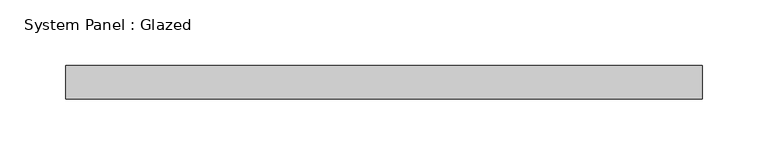
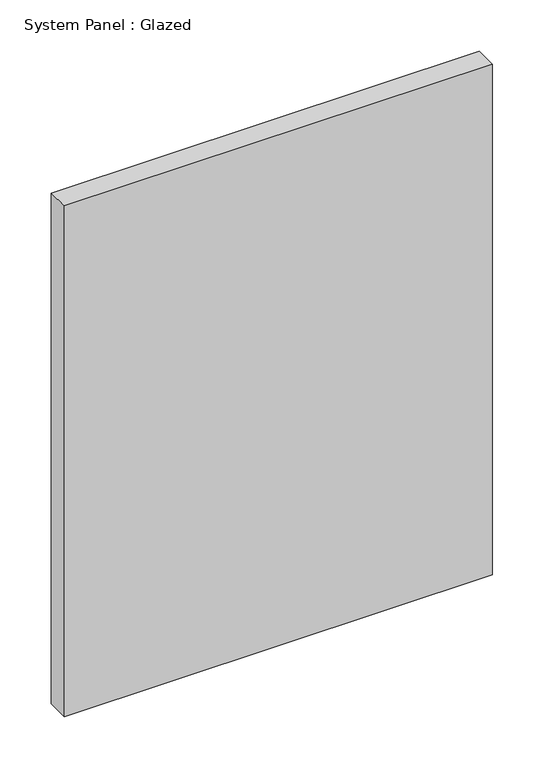
"""IFC4 building model written with IfcOpenShell, lengths in millimetres: plate geometry, System Panel : Glazed."""

from ifc_helpers import new_model, si_unit, origin, origin_with_axes, place, context, project, spatial, polyline, outline, extrude, source, transform, mapped, element, save


def system_panel_glazed_a9204d3a(model_context):
    return source(origin(), model_context, "Body", "SweptSolid", [
        extrude(outline(polyline([(241.3, 19.05), (-241.3, 19.05), (-241.3, 44.45), (241.3, 44.45), (241.3, 19.05)])), origin_with_axes(), (0.0, 0.0, 1.0), 608.6147442),
    ])


if __name__ == "__main__":
    model = new_model("IFC4")
    model_context = context("Model", 3, world=origin())
    ifc_project = project(units=[si_unit("LENGTHUNIT", "METRE", prefix="MILLI")], contexts=[model_context])
    site = spatial("IfcSite", under=ifc_project)
    building = spatial("IfcBuilding", under=site)
    placement = place(None, origin())
    system_panel_glazed_shape = system_panel_glazed_a9204d3a(model_context)
    element("IfcPlate", 1, ObjectType="System Panel : Glazed", at=placement, inside=building, context=model_context, shape_type="MappedRepresentation", body=[
        mapped(system_panel_glazed_shape, transform((0.0, 0.0, 0.0), x_axis=(1.0, 0.0, 0.0), y_axis=(0.0, 1.0, 0.0), z_axis=(0.0, 0.0, 1.0))),
    ])
    save(model, "model.ifc")

# Revit data of these elements
# Type "System Panel : Glazed"
#   Construction Type Id = "GSP4R"
#   Analytic Construction = "1/8 in Pilkington single glazing"
#   Visual Light Transmittance = 0.9
#   Solar Heat Gain Coefficient = 0.86
#   Heat Transfer Coefficient (U) = 1.18115 BTU/(h·ft²·°F)
#   Define Thermal Properties by = 1
# Element 1 (IfcPlate, "System Panel : Glazed")
#   Materials on its faces: "Glass"
# Materials
#   "Glass": class "Glass", colour RGB 0 128 192, transparency 0.75, Description = "Soda Lime Glass", Cost = 0
